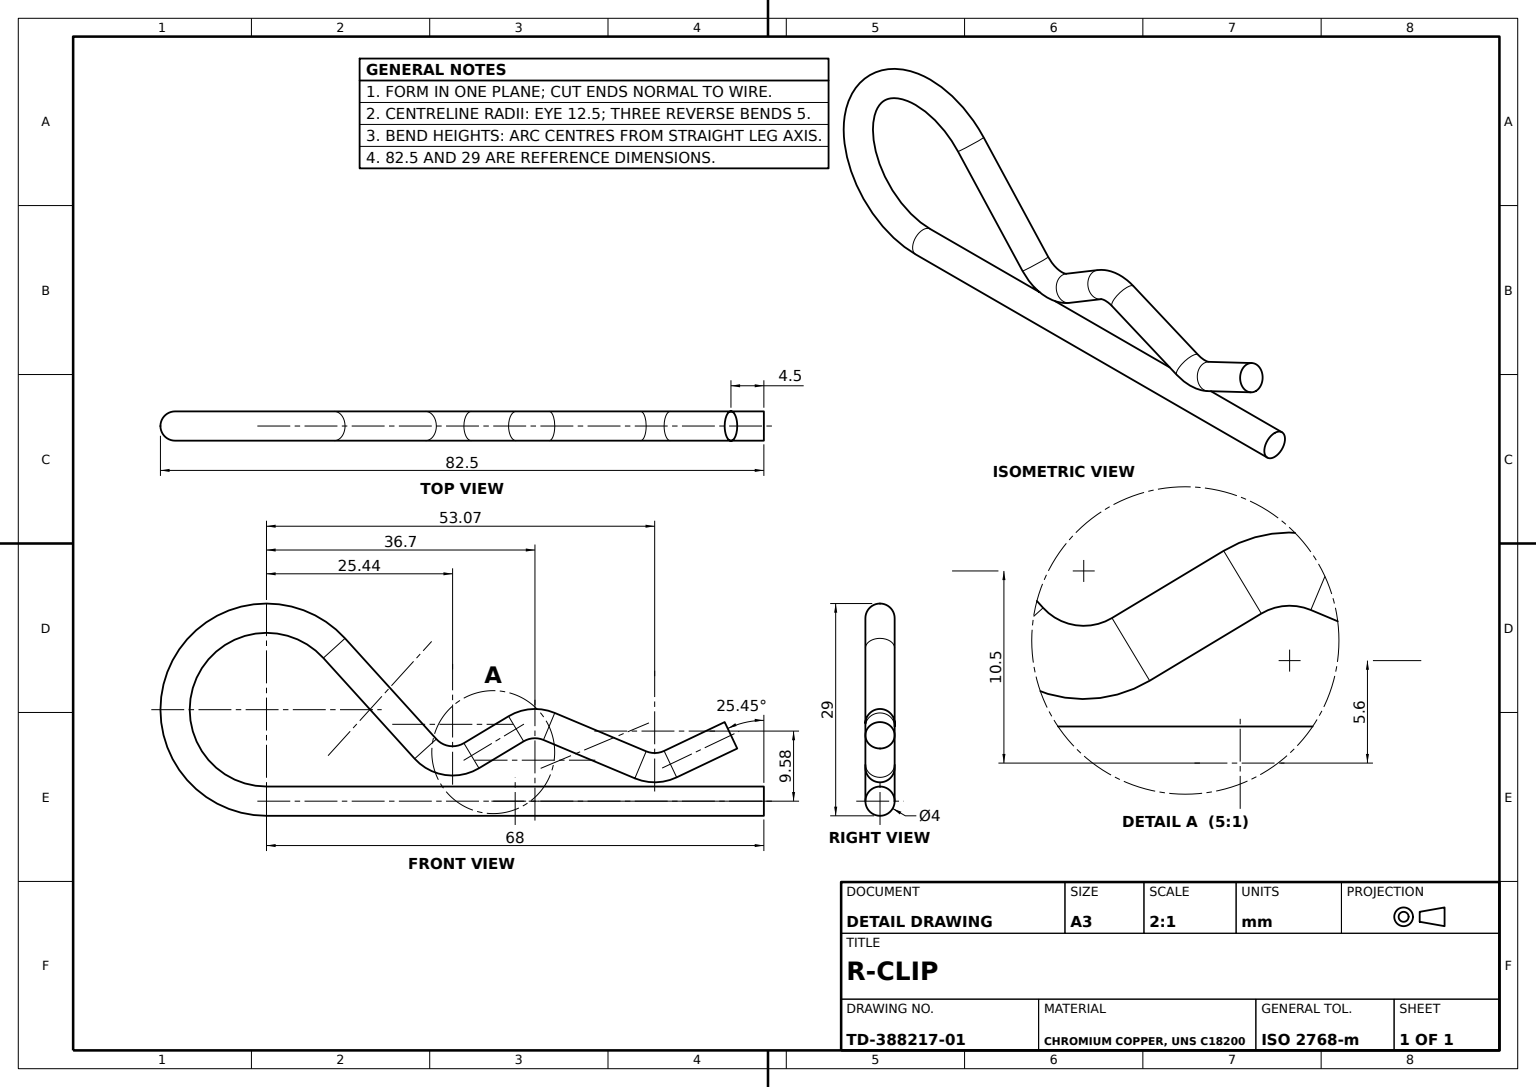
SolidWorks part; units mm, degrees
material "Chromium Copper, UNS C18200"
ref_plane "Front Plane" through (0, 0, 0) normal (0, 0, 1) x (1, 0, 0)
ref_plane "Top Plane" through (0, 0, 0) normal (0, 1, 0) x (1, 0, 0)
ref_plane "Right Plane" through (0, 0, 0) normal (1, 0, 0) x (0, 0, -1)
sketch "Clip Wire Path" plane through (0, 0, 0) normal (0, 0, 1) x (1, 0, 0)
  line L0 (0, 0) -> (-68, 0)
  line L1 (-58.7424, 20.8992) -> (-46.2593, 7.1403)
  line L2 (-39.9804, 6.2145) -> (-33.873, 9.8855)
  line L3 (-29.3623, 10.2104) -> (-16.863, 4.9648)
  line L4 (-12.7798, 5.0603) -> (-4.5, 9)
  line L5 (-68, 0) -> (-68, 31.8553) construction
  arc A0 (-68, 0) -> (-68, 25) centre (-68, 12.5) cw
  arc A1 (-68, 25) -> (-58.7424, 20.8992) centre (-68, 12.5) cw
  arc A2 (-12.7798, 5.0603) -> (-16.863, 4.9648) centre (-14.9281, 9.5753) cw
  arc A3 (-29.3623, 10.2104) -> (-33.873, 9.8855) centre (-31.2971, 5.6) ccw
  arc A4 (-39.9804, 6.2145) -> (-46.2593, 7.1403) centre (-42.5562, 10.5) cw
  point P21 (-14.8, 4.0991)
  point P24 (-31.7, 11.1915)
  point P27 (-43.5, 4.0991)
  dimension "D1" = 12.5
  dimension "D10" = 5
  dimension "D2" = 24.5
  dimension "D3" = 36.3
  dimension "D4" = 53.2
  dimension "D5" = 68
  dimension "D6" = 63.5
  dimension "D7" = 9
  dimension "D8" = 5.6
  dimension "D9" = 10.5
sweep "Wire Sweep Ø4" add path "Clip Wire Path" circular profile diameter 4 parameters "D3"=4
